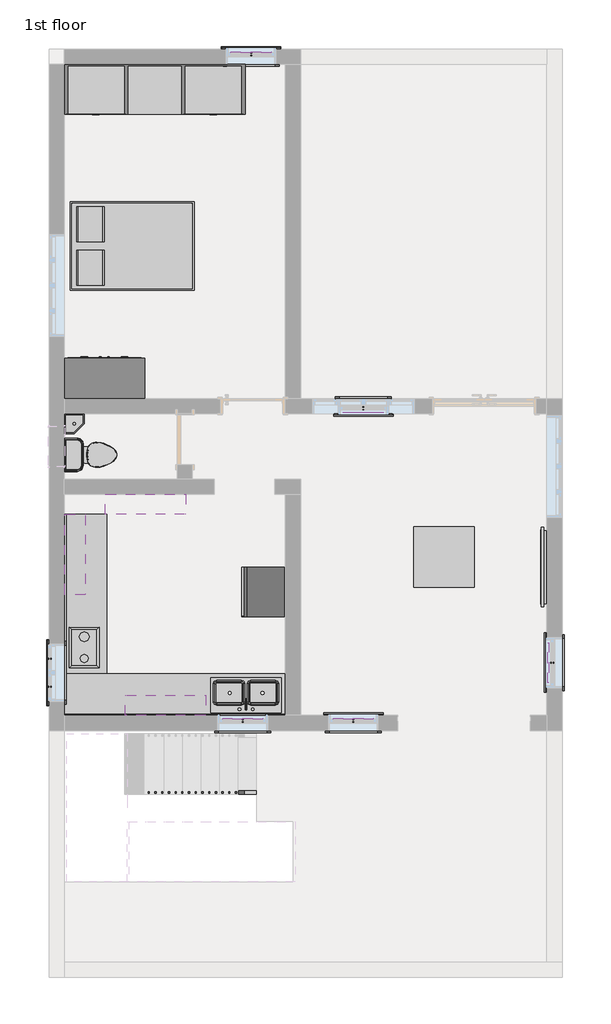
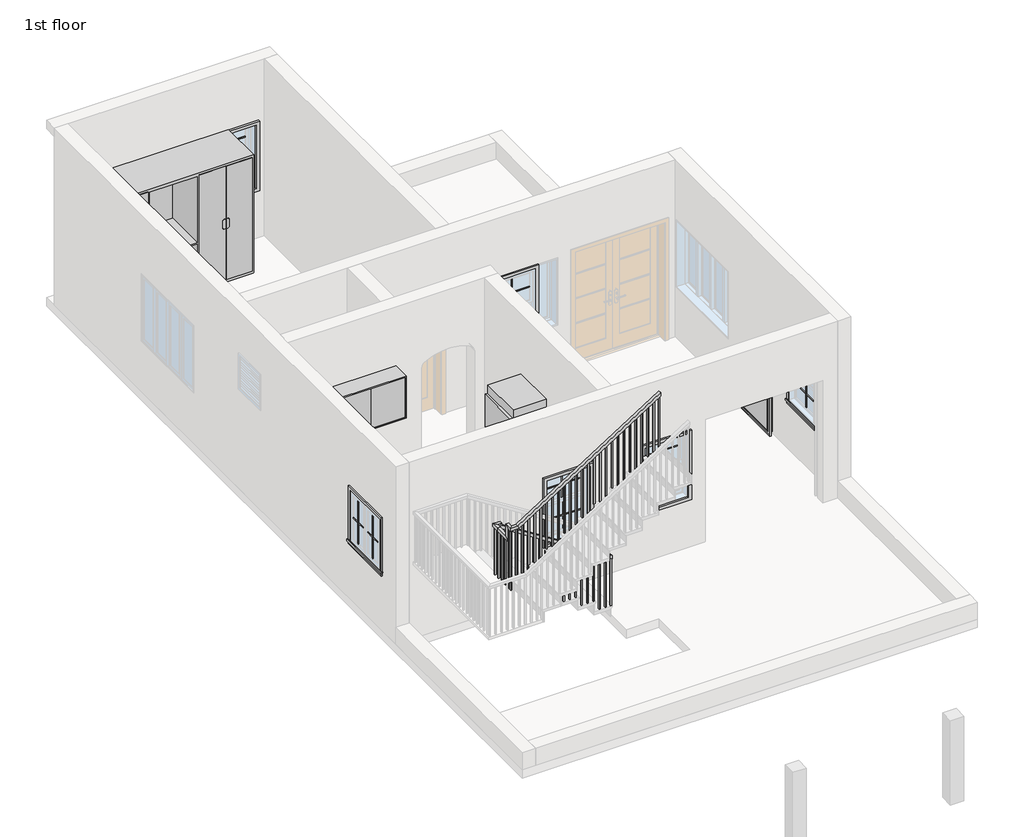
# One storey, part 3 of 3: 26 proxies, 14 furniture elements, 3 flow terminals, 1 railing.
"""IFC4 building model written with IfcOpenShell, lengths in millimetres."""

from ifc_helpers import new_model, si_unit, frame, origin, place, context, project, spatial, polyline, outline, extrude, faceted_brep, transform, mapped, element, save
from components import proxy_3c1fa1d0, muntin_pattern_2x2_muntin_pattern_2x2_b3fe6957, muntin_pattern_2x2_muntin_pattern_2x2_3e0ecaf2, muntin_pattern_2x2_muntin_pattern_2x2_b8ba09c9, muntin_pattern_2x2_muntin_pattern_2x2_d064d722, proxy_76352e5b, trim_window_exterior_flat_with_sill_41619996, trim_window_exterior_flat_with_sill_6cd3ad68, trim_window_exterior_flat_with_sill_e57d6fc0, trim_window_interior_flat_picture_frame_51c85655, trim_window_interior_flat_picture_frame_840a62db, trim_window_interior_flat_picture_frame_50b64344, flow_terminal_080557f2, flow_terminal_a53be723, toilet_domestic_3d_toilet_domestic_3d_ba6479b0, toilet_domestic_3d_toilet_domestic_3d_30431060, furniture_9b4ba0d7, furniture_3428e43d, furniture_97fe820d, furniture_b58f7881, furniture_05b7e736, furniture_e3ff1115, furniture_1f19b6cd, furniture_8a11f05f, furniture_5e39d705, furniture_f491f192, furniture_82e269c4

model = new_model("IFC4")

# Units and contexts
model_context = context("Model", 3, world=origin())
ifc_project = project(units=[si_unit("LENGTHUNIT", "METRE", prefix="MILLI")], contexts=[model_context])

# Site, building, storey
site = spatial("IfcSite", under=ifc_project)
building = spatial("IfcBuilding", under=site)
storey = spatial("IfcBuildingStorey", under=building, Name="1st floor", Elevation=3810.0)

# Proxies
placement = place(None, origin())
proxy_shape = proxy_3c1fa1d0(model_context)
element("IfcBuildingElementProxy", 1, Name="Cook Top-2 Unit : 12\" x 18\" 2", ObjectType="Cook Top-2 Unit : 12\" x 18\" 2", at=placement, inside=storey, context=model_context, shape_type="MappedRepresentation", body=[
    mapped(proxy_shape, transform((28839.5316163, 10560.2732596, 3810.0), x_axis=(1.0, 0.0, 0.0), y_axis=(0.0, 1.0, 0.0), z_axis=(0.0, 0.0, 1.0))),
])
muntin_pattern_2x2_muntin_pattern_2x2_shape = muntin_pattern_2x2_muntin_pattern_2x2_b3fe6957(model_context)
element("IfcBuildingElementProxy", 2, Name="Muntin Pattern_2x2 : Muntin Pattern_2x2", ObjectType="Muntin Pattern_2x2 : Muntin Pattern_2x2", at=placement, inside=storey, context=model_context, shape_type="MappedRepresentation", body=[
    mapped(muntin_pattern_2x2_muntin_pattern_2x2_shape, transform((28391.8566163, 9995.1855552, 4959.35), x_axis=(0.0, 1.0, 0.0), y_axis=(-1.0, 0.0, 0.0), z_axis=(0.0, 0.0, 1.0))),
])
muntin_pattern_2x2_muntin_pattern_2x2_2_shape = muntin_pattern_2x2_muntin_pattern_2x2_3e0ecaf2(model_context)
element("IfcBuildingElementProxy", 3, Name="Muntin Pattern_2x2 : Muntin Pattern_2x2", ObjectType="Muntin Pattern_2x2 : Muntin Pattern_2x2", at=placement, inside=storey, context=model_context, shape_type="MappedRepresentation", body=[
    mapped(muntin_pattern_2x2_muntin_pattern_2x2_2_shape, transform((28391.8566163, 10423.8105552, 4959.35), x_axis=(0.0, -1.0, 0.0), y_axis=(1.0, 0.0, 0.0), z_axis=(0.0, 0.0, 1.0))),
])
muntin_pattern_2x2_muntin_pattern_2x2_3_shape = muntin_pattern_2x2_muntin_pattern_2x2_b8ba09c9(model_context)
element("IfcBuildingElementProxy", 4, Name="Muntin Pattern_2x2 : Muntin Pattern_2x2", ObjectType="Muntin Pattern_2x2 : Muntin Pattern_2x2", at=placement, inside=storey, context=model_context, shape_type="MappedRepresentation", body=[
    mapped(muntin_pattern_2x2_muntin_pattern_2x2_3_shape, transform((32992.4316163, 9526.8730552, 5330.825), x_axis=(1.0, 0.0, 0.0), y_axis=(0.0, 1.0, 0.0), z_axis=(0.0, 0.0, 1.0))),
])
element("IfcBuildingElementProxy", 5, Name="Muntin Pattern_2x2 : Muntin Pattern_2x2", ObjectType="Muntin Pattern_2x2 : Muntin Pattern_2x2", at=placement, inside=storey, context=model_context, shape_type="MappedRepresentation", body=[
    mapped(muntin_pattern_2x2_muntin_pattern_2x2_3_shape, transform((32992.4316163, 9482.4230552, 4800.6), x_axis=(1.0, 0.0, 0.0), y_axis=(0.0, 1.0, 0.0), z_axis=(0.0, 0.0, 1.0))),
])
element("IfcBuildingElementProxy", 6, Name="Muntin Pattern_2x2 : Muntin Pattern_2x2", ObjectType="Muntin Pattern_2x2 : Muntin Pattern_2x2", at=placement, inside=storey, context=model_context, shape_type="MappedRepresentation", body=[
    mapped(muntin_pattern_2x2_muntin_pattern_2x2_3_shape, transform((31316.0316163, 9526.8730552, 5330.825), x_axis=(1.0, 0.0, 0.0), y_axis=(0.0, 1.0, 0.0), z_axis=(0.0, 0.0, 1.0))),
])
element("IfcBuildingElementProxy", 7, Name="Muntin Pattern_2x2 : Muntin Pattern_2x2", ObjectType="Muntin Pattern_2x2 : Muntin Pattern_2x2", at=placement, inside=storey, context=model_context, shape_type="MappedRepresentation", body=[
    mapped(muntin_pattern_2x2_muntin_pattern_2x2_3_shape, transform((31316.0316163, 9482.4230552, 4800.6), x_axis=(1.0, 0.0, 0.0), y_axis=(0.0, 1.0, 0.0), z_axis=(0.0, 0.0, 1.0))),
])
element("IfcBuildingElementProxy", 8, Name="Muntin Pattern_2x2 : Muntin Pattern_2x2", ObjectType="Muntin Pattern_2x2 : Muntin Pattern_2x2", at=placement, inside=storey, context=model_context, shape_type="MappedRepresentation", body=[
    mapped(muntin_pattern_2x2_muntin_pattern_2x2_3_shape, transform((35961.0566163, 10361.8980552, 5330.825), x_axis=(0.0, 1.0, 0.0), y_axis=(-1.0, 0.0, 0.0), z_axis=(0.0, 0.0, 1.0))),
])
element("IfcBuildingElementProxy", 9, Name="Muntin Pattern_2x2 : Muntin Pattern_2x2", ObjectType="Muntin Pattern_2x2 : Muntin Pattern_2x2", at=placement, inside=storey, context=model_context, shape_type="MappedRepresentation", body=[
    mapped(muntin_pattern_2x2_muntin_pattern_2x2_3_shape, transform((36005.5066163, 10361.8980552, 4800.6), x_axis=(0.0, 1.0, 0.0), y_axis=(-1.0, 0.0, 0.0), z_axis=(0.0, 0.0, 1.0))),
])
element("IfcBuildingElementProxy", 10, Name="Muntin Pattern_2x2 : Muntin Pattern_2x2", ObjectType="Muntin Pattern_2x2 : Muntin Pattern_2x2", at=placement, inside=storey, context=model_context, shape_type="MappedRepresentation", body=[
    mapped(muntin_pattern_2x2_muntin_pattern_2x2_3_shape, transform((31443.0316163, 19623.3730552, 5330.825), x_axis=(1.0, 0.0, 0.0), y_axis=(0.0, 1.0, 0.0), z_axis=(0.0, 0.0, 1.0))),
])
element("IfcBuildingElementProxy", 11, Name="Muntin Pattern_2x2 : Muntin Pattern_2x2", ObjectType="Muntin Pattern_2x2 : Muntin Pattern_2x2", at=placement, inside=storey, context=model_context, shape_type="MappedRepresentation", body=[
    mapped(muntin_pattern_2x2_muntin_pattern_2x2_3_shape, transform((31443.0316163, 19578.9230552, 4800.6), x_axis=(1.0, 0.0, 0.0), y_axis=(0.0, 1.0, 0.0), z_axis=(0.0, 0.0, 1.0))),
])
muntin_pattern_2x2_muntin_pattern_2x2_4_shape = muntin_pattern_2x2_muntin_pattern_2x2_d064d722(model_context)
element("IfcBuildingElementProxy", 12, Name="Muntin Pattern_2x2 : Muntin Pattern_2x2", ObjectType="Muntin Pattern_2x2 : Muntin Pattern_2x2", at=placement, inside=storey, context=model_context, shape_type="MappedRepresentation", body=[
    mapped(muntin_pattern_2x2_muntin_pattern_2x2_4_shape, transform((33144.8316163, 14168.7230552, 5330.825), x_axis=(1.0, 0.0, 0.0), y_axis=(0.0, 1.0, 0.0), z_axis=(0.0, 0.0, 1.0))),
])
element("IfcBuildingElementProxy", 13, Name="Muntin Pattern_2x2 : Muntin Pattern_2x2", ObjectType="Muntin Pattern_2x2 : Muntin Pattern_2x2", at=placement, inside=storey, context=model_context, shape_type="MappedRepresentation", body=[
    mapped(muntin_pattern_2x2_muntin_pattern_2x2_4_shape, transform((33144.8316163, 14213.1730552, 4800.6), x_axis=(1.0, 0.0, 0.0), y_axis=(0.0, 1.0, 0.0), z_axis=(0.0, 0.0, 1.0))),
])
proxy_2_shape = proxy_76352e5b(model_context)
element("IfcBuildingElementProxy", 14, Name="Refrigerator-Built-in : 30\" x 24\" LH", ObjectType="Refrigerator-Built-in : 30\" x 24\" LH", at=placement, inside=storey, context=model_context, shape_type="MappedRepresentation", body=[
    mapped(proxy_2_shape, transform((31656.9555878, 11435.0480552, 3810.0), x_axis=(0.0, 1.0, 0.0), y_axis=(-1.0, 0.0, 0.0), z_axis=(0.0, 0.0, 1.0))),
])
trim_window_exterior_flat_with_sill_shape = trim_window_exterior_flat_with_sill_41619996(model_context)
element("IfcBuildingElementProxy", 15, Name="Trim-Window-Exterior-Flat : with Sill", ObjectType="Trim-Window-Exterior-Flat : with Sill", at=placement, inside=storey, context=model_context, shape_type="MappedRepresentation", body=[
    mapped(trim_window_exterior_flat_with_sill_shape, transform((28382.3316163, 10209.4980552, 5803.9), x_axis=(0.0, -1.0, 0.0), y_axis=(0.0, 0.0, 1.0), z_axis=(-1.0, 0.0, 0.0))),
])
trim_window_exterior_flat_with_sill_2_shape = trim_window_exterior_flat_with_sill_6cd3ad68(model_context)
element("IfcBuildingElementProxy", 16, Name="Trim-Window-Exterior-Flat : with Sill", ObjectType="Trim-Window-Exterior-Flat : with Sill", at=placement, inside=storey, context=model_context, shape_type="MappedRepresentation", body=[
    mapped(trim_window_exterior_flat_with_sill_2_shape, transform((32992.4316163, 9561.7980552, 5892.8), x_axis=(-1.0, 0.0, 0.0), y_axis=(0.0, 0.0, 1.0), z_axis=(0.0, 1.0, 0.0))),
])
element("IfcBuildingElementProxy", 17, Name="Trim-Window-Exterior-Flat : with Sill", ObjectType="Trim-Window-Exterior-Flat : with Sill", at=placement, inside=storey, context=model_context, shape_type="MappedRepresentation", body=[
    mapped(trim_window_exterior_flat_with_sill_2_shape, transform((31316.0316163, 9561.7980552, 5892.8), x_axis=(-1.0, 0.0, 0.0), y_axis=(0.0, 0.0, 1.0), z_axis=(0.0, 1.0, 0.0))),
])
element("IfcBuildingElementProxy", 18, Name="Trim-Window-Exterior-Flat : with Sill", ObjectType="Trim-Window-Exterior-Flat : with Sill", at=placement, inside=storey, context=model_context, shape_type="MappedRepresentation", body=[
    mapped(trim_window_exterior_flat_with_sill_2_shape, transform((35926.1316163, 10361.8980552, 5892.8), x_axis=(0.0, -1.0, 0.0), y_axis=(0.0, 0.0, 1.0), z_axis=(-1.0, 0.0, 0.0))),
])
element("IfcBuildingElementProxy", 19, Name="Trim-Window-Exterior-Flat : with Sill", ObjectType="Trim-Window-Exterior-Flat : with Sill", at=placement, inside=storey, context=model_context, shape_type="MappedRepresentation", body=[
    mapped(trim_window_exterior_flat_with_sill_2_shape, transform((31443.0316163, 19658.2980552, 5892.8), x_axis=(-1.0, 0.0, 0.0), y_axis=(0.0, 0.0, 1.0), z_axis=(0.0, 1.0, 0.0))),
])
trim_window_exterior_flat_with_sill_3_shape = trim_window_exterior_flat_with_sill_e57d6fc0(model_context)
element("IfcBuildingElementProxy", 20, Name="Trim-Window-Exterior-Flat : with Sill", ObjectType="Trim-Window-Exterior-Flat : with Sill", at=placement, inside=storey, context=model_context, shape_type="MappedRepresentation", body=[
    mapped(trim_window_exterior_flat_with_sill_3_shape, transform((33144.8316163, 14133.7980552, 5892.8), x_axis=(-1.0, 0.0, 0.0), y_axis=(0.0, 0.0, -1.0), z_axis=(0.0, -1.0, 0.0))),
])
trim_window_interior_flat_picture_frame_shape = trim_window_interior_flat_picture_frame_51c85655(model_context)
element("IfcBuildingElementProxy", 21, Name="Trim-Window-Interior-Flat : Picture Frame", ObjectType="Trim-Window-Interior-Flat : Picture Frame", at=placement, inside=storey, context=model_context, shape_type="MappedRepresentation", body=[
    mapped(trim_window_interior_flat_picture_frame_shape, transform((28610.9316163, 10209.4980552, 5803.9), x_axis=(0.0, 1.0, 0.0), y_axis=(0.0, 0.0, 1.0), z_axis=(1.0, 0.0, 0.0))),
])
trim_window_interior_flat_picture_frame_2_shape = trim_window_interior_flat_picture_frame_840a62db(model_context)
element("IfcBuildingElementProxy", 22, Name="Trim-Window-Interior-Flat : Picture Frame", ObjectType="Trim-Window-Interior-Flat : Picture Frame", at=placement, inside=storey, context=model_context, shape_type="MappedRepresentation", body=[
    mapped(trim_window_interior_flat_picture_frame_2_shape, transform((32992.4316163, 9333.1980552, 5892.8), x_axis=(1.0, 0.0, 0.0), y_axis=(0.0, 0.0, 1.0), z_axis=(0.0, -1.0, 0.0))),
])
element("IfcBuildingElementProxy", 23, Name="Trim-Window-Interior-Flat : Picture Frame", ObjectType="Trim-Window-Interior-Flat : Picture Frame", at=placement, inside=storey, context=model_context, shape_type="MappedRepresentation", body=[
    mapped(trim_window_interior_flat_picture_frame_2_shape, transform((31316.0316163, 9333.1980552, 5892.8), x_axis=(1.0, 0.0, 0.0), y_axis=(0.0, 0.0, 1.0), z_axis=(0.0, -1.0, 0.0))),
])
element("IfcBuildingElementProxy", 24, Name="Trim-Window-Interior-Flat : Picture Frame", ObjectType="Trim-Window-Interior-Flat : Picture Frame", at=placement, inside=storey, context=model_context, shape_type="MappedRepresentation", body=[
    mapped(trim_window_interior_flat_picture_frame_2_shape, transform((36154.7316163, 10361.8980552, 5892.8), x_axis=(0.0, 1.0, 0.0), y_axis=(0.0, 0.0, 1.0), z_axis=(1.0, 0.0, 0.0))),
])
element("IfcBuildingElementProxy", 25, Name="Trim-Window-Interior-Flat : Picture Frame", ObjectType="Trim-Window-Interior-Flat : Picture Frame", at=placement, inside=storey, context=model_context, shape_type="MappedRepresentation", body=[
    mapped(trim_window_interior_flat_picture_frame_2_shape, transform((31443.0316163, 19429.6980552, 5892.8), x_axis=(1.0, 0.0, 0.0), y_axis=(0.0, 0.0, 1.0), z_axis=(0.0, -1.0, 0.0))),
])
trim_window_interior_flat_picture_frame_3_shape = trim_window_interior_flat_picture_frame_50b64344(model_context)
element("IfcBuildingElementProxy", 26, Name="Trim-Window-Interior-Flat : Picture Frame", ObjectType="Trim-Window-Interior-Flat : Picture Frame", at=placement, inside=storey, context=model_context, shape_type="MappedRepresentation", body=[
    mapped(trim_window_interior_flat_picture_frame_3_shape, transform((33144.8316163, 14362.3980552, 5892.8), x_axis=(1.0, 0.0, 0.0), y_axis=(0.0, 0.0, -1.0), z_axis=(0.0, 1.0, 0.0))),
])

# Flow terminals
flow_terminal_shape = flow_terminal_080557f2(model_context)
element("IfcFlowTerminal", 27, ObjectType="Sink - Mop : 28\"x28\" 2", at=placement, inside=storey, context=model_context, shape_type="MappedRepresentation", body=[
    mapped(flow_terminal_shape, transform((28610.9316163, 14133.7980552, 4724.4), x_axis=(1.0, 0.0, 0.0), y_axis=(0.0, 1.0, 0.0), z_axis=(0.0, 0.0, 1.0))),
])
flow_terminal_2_shape = flow_terminal_a53be723(model_context)
element("IfcFlowTerminal", 28, ObjectType="Sink Kitchen-Double : 42\" x 21\"", at=placement, inside=storey, context=model_context, shape_type="MappedRepresentation", body=[
    mapped(flow_terminal_2_shape, transform((31382.5208569, 9868.9434563, 3810.0), x_axis=(-1.0, 0.0, 0.0), y_axis=(0.0, -1.0, 0.0), z_axis=(0.0, 0.0, 1.0))),
])
toilet_domestic_3d_toilet_domestic_3d_shape = toilet_domestic_3d_toilet_domestic_3d_ba6479b0(model_context)
toilet_domestic_3d_toilet_domestic_3d_2_shape = toilet_domestic_3d_toilet_domestic_3d_30431060(model_context)
element("IfcFlowTerminal", 29, ObjectType="Toilet-Domestic-3D : Toilet-Domestic-3D", at=placement, inside=storey, context=model_context, shape_type="MappedRepresentation", body=[
    mapped(toilet_domestic_3d_toilet_domestic_3d_shape, transform((29105.6276437, 13511.4980552, 3810.0), x_axis=(0.0, 1.0, 0.0), y_axis=(-1.0, 0.0, 0.0), z_axis=(0.0, 0.0, 1.0))),
    mapped(toilet_domestic_3d_toilet_domestic_3d_2_shape, transform((29105.6276437, 13511.4980552, 3810.0), x_axis=(0.0, 1.0, 0.0), y_axis=(-1.0, 0.0, 0.0), z_axis=(0.0, 0.0, 1.0))),
])

# Furniture
furniture_shape = furniture_9b4ba0d7(model_context)
element("IfcFurniture", 30, ObjectType="36\"", at=placement, inside=storey, context=model_context, shape_type="MappedRepresentation", body=[
    mapped(furniture_shape, transform((28623.6316163, 12133.8603503, 3810.0), x_axis=(0.0, 1.0, 0.0), y_axis=(-1.0, 0.0, 0.0), z_axis=(0.0, 0.0, 1.0))),
])
furniture_2_shape = furniture_3428e43d(model_context)
element("IfcFurniture", 31, ObjectType="48\"", at=placement, inside=storey, context=model_context, shape_type="MappedRepresentation", body=[
    mapped(furniture_2_shape, transform((30238.4765763, 9561.7980552, 3810.0), x_axis=(-1.0, 0.0, 0.0), y_axis=(0.0, -1.0, 0.0), z_axis=(0.0, 0.0, 1.0))),
])
element("IfcFurniture", 32, ObjectType="48\"", at=placement, inside=storey, context=model_context, shape_type="MappedRepresentation", body=[
    mapped(furniture_2_shape, transform((28623.6316163, 10994.9530952, 3810.0), x_axis=(0.0, 1.0, 0.0), y_axis=(-1.0, 0.0, 0.0), z_axis=(0.0, 0.0, 1.0))),
])
furniture_3_shape = furniture_97fe820d(model_context)
element("IfcFurniture", 33, ObjectType="Base Cabinet-Corner Unit-Square : 36\"", at=placement, inside=storey, context=model_context, shape_type="MappedRepresentation", body=[
    mapped(furniture_3_shape, transform((29150.3693213, 9561.7980552, 3810.0), x_axis=(-1.0, 0.0, 0.0), y_axis=(0.0, -1.0, 0.0), z_axis=(0.0, 0.0, 1.0))),
])
furniture_4_shape = furniture_b58f7881(model_context)
element("IfcFurniture", 34, ObjectType="Bed-Box : Double 53\" x 74\"", at=placement, inside=storey, context=model_context, shape_type="MappedRepresentation", body=[
    mapped(furniture_4_shape, transform((29405.2021081, 16334.6455962, 3810.0), x_axis=(0.0, 1.0, 0.0), y_axis=(-1.0, 0.0, 0.0), z_axis=(0.0, 0.0, 1.0))),
])
furniture_5_shape = furniture_05b7e736(model_context)
element("IfcFurniture", 35, ObjectType="Counter Top : 24\" Depth", at=placement, inside=storey, context=model_context, shape_type="MappedRepresentation", body=[
    mapped(furniture_5_shape, transform((28623.6316163, 11397.2603503, 3810.0), x_axis=(0.0, 1.0, 0.0), y_axis=(-1.0, 0.0, 0.0), z_axis=(0.0, 0.0, 1.0))),
])
furniture_6_shape = furniture_e3ff1115(model_context)
element("IfcFurniture", 36, ObjectType="Counter Top w Sink : 24\" Depth", at=placement, inside=storey, context=model_context, shape_type="MappedRepresentation", body=[
    mapped(furniture_6_shape, transform((30775.9693213, 9561.7980552, 3810.0), x_axis=(-1.0, 0.0, 0.0), y_axis=(0.0, -1.0, 0.0), z_axis=(0.0, 0.0, 1.0))),
])
furniture_7_shape = furniture_1f19b6cd(model_context)
element("IfcFurniture", 37, ObjectType="Entertainment Center.0001 : 96\" x 84\" x 30\"", at=placement, inside=storey, context=model_context, shape_type="MappedRepresentation", body=[
    mapped(furniture_7_shape, transform((29982.5316163, 19455.0980552, 3810.0), x_axis=(1.0, 0.0, 0.0), y_axis=(0.0, 1.0, 0.0), z_axis=(0.0, 0.0, 1.0))),
])
furniture_8_shape = furniture_8a11f05f(model_context)
element("IfcFurniture", 38, ObjectType="Table-Rectangular : 36\" x 36\" 2", at=placement, inside=storey, context=model_context, shape_type="MappedRepresentation", body=[
    mapped(furniture_8_shape, transform((34364.0316163, 11962.0980552, 3810.0), x_axis=(1.0, 0.0, 0.0), y_axis=(0.0, 1.0, 0.0), z_axis=(0.0, 0.0, 1.0))),
])
furniture_9_shape = furniture_5e39d705(model_context)
element("IfcFurniture", 39, ObjectType="Television-Plasma : 50\"", at=placement, inside=storey, context=model_context, shape_type="MappedRepresentation", body=[
    mapped(furniture_9_shape, transform((35926.1316163, 11866.8480552, 3810.0), x_axis=(0.0, -1.0, 0.0), y_axis=(1.0, 0.0, 0.0), z_axis=(0.0, 0.0, 1.0))),
])
furniture_10_shape = furniture_f491f192(model_context)
element("IfcFurniture", 40, ObjectType="Upper Cabinet-Pass-Thru w Glass : 48\" x 30\" x 12\"", at=placement, inside=storey, context=model_context, shape_type="MappedRepresentation", body=[
    mapped(furniture_10_shape, transform((28623.6316163, 11981.4603503, 3810.0), x_axis=(0.0, 1.0, 0.0), y_axis=(-1.0, 0.0, 0.0), z_axis=(0.0, 0.0, 1.0))),
])
element("IfcFurniture", 41, ObjectType="Upper Cabinet-Pass-Thru w Glass : 48\" x 30\" x 12\"", at=placement, inside=storey, context=model_context, shape_type="MappedRepresentation", body=[
    mapped(furniture_10_shape, transform((29861.5693213, 12609.7980552, 3810.0), x_axis=(-1.0, 0.0, 0.0), y_axis=(0.0, -1.0, 0.0), z_axis=(0.0, 0.0, 1.0))),
])
element("IfcFurniture", 42, ObjectType="Upper Cabinet-Pass-Thru w Glass : 48\" x 30\" x 12\"", at=placement, inside=storey, context=model_context, shape_type="MappedRepresentation", body=[
    mapped(furniture_10_shape, transform((30166.3693213, 9561.7980552, 3810.0), x_axis=(-1.0, 0.0, 0.0), y_axis=(0.0, -1.0, 0.0), z_axis=(0.0, 0.0, 1.0))),
])
furniture_11_shape = furniture_82e269c4(model_context)
element("IfcFurniture", 43, ObjectType="Wardrobe : 48\" x 72\" x 24\"", at=placement, inside=storey, context=model_context, shape_type="MappedRepresentation", body=[
    mapped(furniture_11_shape, transform((28951.3383565, 14083.4592456, 3810.0), x_axis=(-1.0, 0.0, 0.0), y_axis=(0.0, -1.0, 0.0), z_axis=(0.0, 0.0, 1.0))),
])

# Railing
element("IfcRailing", 44, ObjectType="Handrail - Rectangular", at=placement, inside=storey, context=model_context, shape_type="SolidModel", body=[
    faceted_brep([(31519.2316163, 8367.9980552, 4902.2), (31519.2316163, 8367.9980552, 4841.986276), (31519.2316163, 8418.7980552, 4841.986276), (31519.2316163, 8418.7980552, 4902.2), (29639.6316163, 8367.9980552, 6098.3090909), (29588.8316163, 8367.9980552, 6070.4226396), (29588.8316163, 8418.7980552, 6070.4226396), (29639.6316163, 8418.7980552, 6098.3090909), (29639.6316163, 8367.9980552, 6146.8), (29588.8316163, 8367.9980552, 6096.0), (29588.8316163, 8418.7980552, 6096.0), (29639.6316163, 8418.7980552, 6146.8), (29563.4316163, 8367.9980552, 6146.8), (29563.4316163, 8367.9980552, 6096.0), (29512.6316163, 8418.7980552, 6096.0), (29512.6316163, 8418.7980552, 6146.8), (29563.4316163, 8291.7980552, 6146.8), (29563.4316163, 8291.7980552, 6096.0), (29512.6316163, 8291.7980552, 6096.0), (29512.6316163, 8291.7980552, 6146.8), (29563.4316163, 8031.4480552, 6146.8), (29563.4316163, 7980.6480552, 6096.0), (29512.6316163, 7980.6480552, 6096.0), (29512.6316163, 8031.4480552, 6146.8), (29563.4316163, 8031.4480552, 6373.0909091), (29563.4316163, 7980.6480552, 6322.2909091), (29512.6316163, 7980.6480552, 6322.2909091), (29512.6316163, 8031.4480552, 6373.0909091), (29563.4316163, 7955.2480552, 6373.0909091), (29563.4316163, 7955.2480552, 6322.2909091), (29512.6316163, 7904.4480552, 6322.2909091), (29512.6316163, 7904.4480552, 6373.0909091), (29639.6316163, 7955.2480552, 6373.0909091), (29654.4246113, 7955.2480552, 6322.2909091), (29654.4246113, 7904.4480552, 6322.2909091), (29639.6316163, 7904.4480552, 6373.0909091), (32078.0316163, 7955.2480552, 7924.8), (32078.0316163, 7904.4480552, 7924.8), (32078.0316163, 7904.4480552, 7864.586276), (32078.0316163, 7955.2480552, 7864.586276)], [[[0, 1, 2, 3]], [[1, 0, 4, 5]], [[2, 1, 5, 6]], [[3, 2, 6, 7]], [[0, 3, 7, 4]], [[5, 4, 8, 9]], [[6, 5, 9, 10]], [[7, 6, 10, 11]], [[4, 7, 11, 8]], [[9, 8, 12, 13]], [[10, 9, 13, 14]], [[11, 10, 14, 15]], [[8, 11, 15, 12]], [[13, 12, 16, 17]], [[14, 13, 17, 18]], [[15, 14, 18, 19]], [[12, 15, 19, 16]], [[17, 16, 20, 21]], [[18, 17, 21, 22]], [[19, 18, 22, 23]], [[16, 19, 23, 20]], [[21, 20, 24, 25]], [[22, 21, 25, 26]], [[23, 22, 26, 27]], [[20, 23, 27, 24]], [[25, 24, 28, 29]], [[26, 25, 29, 30]], [[27, 26, 30, 31]], [[24, 27, 31, 28]], [[29, 28, 32, 33]], [[30, 29, 33, 34]], [[31, 30, 34, 35]], [[28, 31, 35, 32]], [[36, 37, 38, 39]], [[33, 32, 36, 39]], [[34, 33, 39, 38]], [[35, 34, 38, 37]], [[32, 35, 37, 36]]]),
    extrude(outline(polyline([(7793.8703669, 31966.9066163), (6832.6, 31966.9066163), (6832.6, 31985.9566163), (7805.9930941, 31985.9566163), (7793.8703669, 31966.9066163)])), frame((0.0, 7920.3230552, 0.0), z_axis=(0.0, 1.0, 0.0), x_axis=(0.0, 0.0, 1.0)), (0.0, 0.0, 1.0), 19.05),
    extrude(outline(polyline([(7729.2158214, 31865.3066163), (6832.6, 31865.3066163), (6832.6, 31884.3566163), (7741.3385487, 31884.3566163), (7729.2158214, 31865.3066163)])), frame((0.0, 7920.3230552, 0.0), z_axis=(0.0, 1.0, 0.0), x_axis=(0.0, 0.0, 1.0)), (0.0, 0.0, 1.0), 19.05),
    extrude(outline(polyline([(7664.561276, 31763.7066163), (6654.8, 31763.7066163), (6654.8, 31782.7566163), (7676.6840032, 31782.7566163), (7664.561276, 31763.7066163)])), frame((0.0, 7920.3230552, 0.0), z_axis=(0.0, 1.0, 0.0), x_axis=(0.0, 0.0, 1.0)), (0.0, 0.0, 1.0), 19.05),
    extrude(outline(polyline([(7599.9067305, 31662.1066163), (6654.8, 31662.1066163), (6654.8, 31681.1566163), (7612.0294578, 31681.1566163), (7599.9067305, 31662.1066163)])), frame((0.0, 7920.3230552, 0.0), z_axis=(0.0, 1.0, 0.0), x_axis=(0.0, 0.0, 1.0)), (0.0, 0.0, 1.0), 19.05),
    extrude(outline(polyline([(7535.2521851, 31560.5066163), (6654.8, 31560.5066163), (6654.8, 31579.5566163), (7547.3749123, 31579.5566163), (7535.2521851, 31560.5066163)])), frame((0.0, 7920.3230552, 0.0), z_axis=(0.0, 1.0, 0.0), x_axis=(0.0, 0.0, 1.0)), (0.0, 0.0, 1.0), 19.05),
    extrude(outline(polyline([(7470.5976396, 31458.9066163), (6477.0, 31458.9066163), (6477.0, 31477.9566163), (7482.7203669, 31477.9566163), (7470.5976396, 31458.9066163)])), frame((0.0, 7920.3230552, 0.0), z_axis=(0.0, 1.0, 0.0), x_axis=(0.0, 0.0, 1.0)), (0.0, 0.0, 1.0), 19.05),
    extrude(outline(polyline([(7405.9430941, 31357.3066163), (6477.0, 31357.3066163), (6477.0, 31376.3566163), (7418.0658214, 31376.3566163), (7405.9430941, 31357.3066163)])), frame((0.0, 7920.3230552, 0.0), z_axis=(0.0, 1.0, 0.0), x_axis=(0.0, 0.0, 1.0)), (0.0, 0.0, 1.0), 19.05),
    extrude(outline(polyline([(7341.2885487, 31255.7066163), (6477.0, 31255.7066163), (6477.0, 31274.7566163), (7353.411276, 31274.7566163), (7341.2885487, 31255.7066163)])), frame((0.0, 7920.3230552, 0.0), z_axis=(0.0, 1.0, 0.0), x_axis=(0.0, 0.0, 1.0)), (0.0, 0.0, 1.0), 19.05),
    extrude(outline(polyline([(7276.6340032, 31154.1066163), (6299.2, 31154.1066163), (6299.2, 31173.1566163), (7288.7567305, 31173.1566163), (7276.6340032, 31154.1066163)])), frame((0.0, 7920.3230552, 0.0), z_axis=(0.0, 1.0, 0.0), x_axis=(0.0, 0.0, 1.0)), (0.0, 0.0, 1.0), 19.05),
    extrude(outline(polyline([(7211.9794578, 31052.5066163), (6299.2, 31052.5066163), (6299.2, 31071.5566163), (7224.1021851, 31071.5566163), (7211.9794578, 31052.5066163)])), frame((0.0, 7920.3230552, 0.0), z_axis=(0.0, 1.0, 0.0), x_axis=(0.0, 0.0, 1.0)), (0.0, 0.0, 1.0), 19.05),
    extrude(outline(polyline([(7147.3249123, 30950.9066163), (6299.2, 30950.9066163), (6299.2, 30969.9566163), (7159.4476396, 30969.9566163), (7147.3249123, 30950.9066163)])), frame((0.0, 7920.3230552, 0.0), z_axis=(0.0, 1.0, 0.0), x_axis=(0.0, 0.0, 1.0)), (0.0, 0.0, 1.0), 19.05),
    extrude(outline(polyline([(7082.6703669, 30849.3066163), (6121.4, 30849.3066163), (6121.4, 30868.3566163), (7094.7930941, 30868.3566163), (7082.6703669, 30849.3066163)])), frame((0.0, 7920.3230552, 0.0), z_axis=(0.0, 1.0, 0.0), x_axis=(0.0, 0.0, 1.0)), (0.0, 0.0, 1.0), 19.05),
    extrude(outline(polyline([(7018.0158214, 30747.7066163), (6121.4, 30747.7066163), (6121.4, 30766.7566163), (7030.1385487, 30766.7566163), (7018.0158214, 30747.7066163)])), frame((0.0, 7920.3230552, 0.0), z_axis=(0.0, 1.0, 0.0), x_axis=(0.0, 0.0, 1.0)), (0.0, 0.0, 1.0), 19.05),
    extrude(outline(polyline([(6953.361276, 30646.1066163), (5943.6, 30646.1066163), (5943.6, 30665.1566163), (6965.4840032, 30665.1566163), (6953.361276, 30646.1066163)])), frame((0.0, 7920.3230552, 0.0), z_axis=(0.0, 1.0, 0.0), x_axis=(0.0, 0.0, 1.0)), (0.0, 0.0, 1.0), 19.05),
    extrude(outline(polyline([(6888.7067305, 30544.5066163), (5943.6, 30544.5066163), (5943.6, 30563.5566163), (6900.8294578, 30563.5566163), (6888.7067305, 30544.5066163)])), frame((0.0, 7920.3230552, 0.0), z_axis=(0.0, 1.0, 0.0), x_axis=(0.0, 0.0, 1.0)), (0.0, 0.0, 1.0), 19.05),
    extrude(outline(polyline([(6824.0521851, 30442.9066163), (5943.6, 30442.9066163), (5943.6, 30461.9566163), (6836.1749123, 30461.9566163), (6824.0521851, 30442.9066163)])), frame((0.0, 7920.3230552, 0.0), z_axis=(0.0, 1.0, 0.0), x_axis=(0.0, 0.0, 1.0)), (0.0, 0.0, 1.0), 19.05),
    extrude(outline(polyline([(6759.3976396, 30341.3066163), (5765.8, 30341.3066163), (5765.8, 30360.3566163), (6771.5203669, 30360.3566163), (6759.3976396, 30341.3066163)])), frame((0.0, 7920.3230552, 0.0), z_axis=(0.0, 1.0, 0.0), x_axis=(0.0, 0.0, 1.0)), (0.0, 0.0, 1.0), 19.05),
    extrude(outline(polyline([(6694.7430941, 30239.7066163), (5765.8, 30239.7066163), (5765.8, 30258.7566163), (6706.8658214, 30258.7566163), (6694.7430941, 30239.7066163)])), frame((0.0, 7920.3230552, 0.0), z_axis=(0.0, 1.0, 0.0), x_axis=(0.0, 0.0, 1.0)), (0.0, 0.0, 1.0), 19.05),
    extrude(outline(polyline([(6630.0885487, 30138.1066163), (5765.8, 30138.1066163), (5765.8, 30157.1566163), (6642.211276, 30157.1566163), (6630.0885487, 30138.1066163)])), frame((0.0, 7920.3230552, 0.0), z_axis=(0.0, 1.0, 0.0), x_axis=(0.0, 0.0, 1.0)), (0.0, 0.0, 1.0), 19.05),
    extrude(outline(polyline([(6565.4340032, 30036.5066163), (5588.0, 30036.5066163), (5588.0, 30055.5566163), (6577.5567305, 30055.5566163), (6565.4340032, 30036.5066163)])), frame((0.0, 7920.3230552, 0.0), z_axis=(0.0, 1.0, 0.0), x_axis=(0.0, 0.0, 1.0)), (0.0, 0.0, 1.0), 19.05),
    extrude(outline(polyline([(6500.7794578, 29934.9066163), (5588.0, 29934.9066163), (5588.0, 29953.9566163), (6512.9021851, 29953.9566163), (6500.7794578, 29934.9066163)])), frame((0.0, 7920.3230552, 0.0), z_axis=(0.0, 1.0, 0.0), x_axis=(0.0, 0.0, 1.0)), (0.0, 0.0, 1.0), 19.05),
    extrude(outline(polyline([(6436.1249123, 29833.3066163), (5588.0, 29833.3066163), (5588.0, 29852.3566163), (6448.2476396, 29852.3566163), (6436.1249123, 29833.3066163)])), frame((0.0, 7920.3230552, 0.0), z_axis=(0.0, 1.0, 0.0), x_axis=(0.0, 0.0, 1.0)), (0.0, 0.0, 1.0), 19.05),
    extrude(outline(polyline([(6371.4703669, 29731.7066163), (5410.2, 29731.7066163), (5410.2, 29750.7566163), (6383.5930941, 29750.7566163), (6371.4703669, 29731.7066163)])), frame((0.0, 7920.3230552, 0.0), z_axis=(0.0, 1.0, 0.0), x_axis=(0.0, 0.0, 1.0)), (0.0, 0.0, 1.0), 19.05),
    extrude(outline(polyline([(6306.8158214, 29630.1066163), (5410.2, 29630.1066163), (5410.2, 29649.1566163), (6318.9385487, 29649.1566163), (6306.8158214, 29630.1066163)])), frame((0.0, 7920.3230552, 0.0), z_axis=(0.0, 1.0, 0.0), x_axis=(0.0, 0.0, 1.0)), (0.0, 0.0, 1.0), 19.05),
    extrude(outline(polyline([(29547.5566163, 7996.5230552), (29547.5566163, 7977.4730552), (29528.5066163, 7977.4730552), (29528.5066163, 7996.5230552), (29547.5566163, 7996.5230552)])), frame((0.0, 0.0, 5232.4), z_axis=(0.0, 0.0, 1.0), x_axis=(1.0, 0.0, 0.0)), (0.0, 0.0, 1.0), 1089.8909091),
    extrude(outline(polyline([(29547.5566163, 8098.1230552), (29547.5566163, 8079.0730552), (29528.5066163, 8079.0730552), (29528.5066163, 8098.1230552), (29547.5566163, 8098.1230552)])), frame((0.0, 0.0, 5232.4), z_axis=(0.0, 0.0, 1.0), x_axis=(1.0, 0.0, 0.0)), (0.0, 0.0, 1.0), 863.6),
    extrude(outline(polyline([(29547.5566163, 8199.7230552), (29547.5566163, 8180.6730552), (29528.5066163, 8180.6730552), (29528.5066163, 8199.7230552), (29547.5566163, 8199.7230552)])), frame((0.0, 0.0, 5232.4), z_axis=(0.0, 0.0, 1.0), x_axis=(1.0, 0.0, 0.0)), (0.0, 0.0, 1.0), 863.6),
    extrude(outline(polyline([(29547.5566163, 8301.3230552), (29547.5566163, 8282.2730552), (29528.5066163, 8282.2730552), (29528.5066163, 8301.3230552), (29547.5566163, 8301.3230552)])), frame((0.0, 0.0, 5232.4), z_axis=(0.0, 0.0, 1.0), x_axis=(1.0, 0.0, 0.0)), (0.0, 0.0, 1.0), 863.6),
    extrude(outline(polyline([(29598.3566163, 8383.8730552), (29579.3066163, 8383.8730552), (29579.3066163, 8402.9230552), (29598.3566163, 8402.9230552), (29598.3566163, 8383.8730552)])), frame((0.0, 0.0, 5054.6), z_axis=(0.0, 0.0, 1.0), x_axis=(1.0, 0.0, 0.0)), (0.0, 0.0, 1.0), 1041.4),
    extrude(outline(polyline([(6011.8294578, 29680.9066163), (5054.6, 29680.9066163), (5054.6, 29699.9566163), (5999.7067305, 29699.9566163), (6011.8294578, 29680.9066163)])), frame((0.0, 8383.8730552, 0.0), z_axis=(0.0, 1.0, 0.0), x_axis=(0.0, 0.0, 1.0)), (0.0, 0.0, 1.0), 19.05),
    extrude(outline(polyline([(5947.1749123, 29782.5066163), (5054.6, 29782.5066163), (5054.6, 29801.5566163), (5935.0521851, 29801.5566163), (5947.1749123, 29782.5066163)])), frame((0.0, 8383.8730552, 0.0), z_axis=(0.0, 1.0, 0.0), x_axis=(0.0, 0.0, 1.0)), (0.0, 0.0, 1.0), 19.05),
    extrude(outline(polyline([(5882.5203669, 29884.1066163), (4876.8, 29884.1066163), (4876.8, 29903.1566163), (5870.3976396, 29903.1566163), (5882.5203669, 29884.1066163)])), frame((0.0, 8383.8730552, 0.0), z_axis=(0.0, 1.0, 0.0), x_axis=(0.0, 0.0, 1.0)), (0.0, 0.0, 1.0), 19.05),
    extrude(outline(polyline([(5817.8658214, 29985.7066163), (4876.8, 29985.7066163), (4876.8, 30004.7566163), (5805.7430941, 30004.7566163), (5817.8658214, 29985.7066163)])), frame((0.0, 8383.8730552, 0.0), z_axis=(0.0, 1.0, 0.0), x_axis=(0.0, 0.0, 1.0)), (0.0, 0.0, 1.0), 19.05),
    extrude(outline(polyline([(5753.211276, 30087.3066163), (4876.8, 30087.3066163), (4876.8, 30106.3566163), (5741.0885487, 30106.3566163), (5753.211276, 30087.3066163)])), frame((0.0, 8383.8730552, 0.0), z_axis=(0.0, 1.0, 0.0), x_axis=(0.0, 0.0, 1.0)), (0.0, 0.0, 1.0), 19.05),
    extrude(outline(polyline([(5688.5567305, 30188.9066163), (4699.0, 30188.9066163), (4699.0, 30207.9566163), (5676.4340032, 30207.9566163), (5688.5567305, 30188.9066163)])), frame((0.0, 8383.8730552, 0.0), z_axis=(0.0, 1.0, 0.0), x_axis=(0.0, 0.0, 1.0)), (0.0, 0.0, 1.0), 19.05),
    extrude(outline(polyline([(5623.9021851, 30290.5066163), (4699.0, 30290.5066163), (4699.0, 30309.5566163), (5611.7794578, 30309.5566163), (5623.9021851, 30290.5066163)])), frame((0.0, 8383.8730552, 0.0), z_axis=(0.0, 1.0, 0.0), x_axis=(0.0, 0.0, 1.0)), (0.0, 0.0, 1.0), 19.05),
    extrude(outline(polyline([(5559.2476396, 30392.1066163), (4699.0, 30392.1066163), (4699.0, 30411.1566163), (5547.1249123, 30411.1566163), (5559.2476396, 30392.1066163)])), frame((0.0, 8383.8730552, 0.0), z_axis=(0.0, 1.0, 0.0), x_axis=(0.0, 0.0, 1.0)), (0.0, 0.0, 1.0), 19.05),
    extrude(outline(polyline([(5494.5930941, 30493.7066163), (4521.2, 30493.7066163), (4521.2, 30512.7566163), (5482.4703669, 30512.7566163), (5494.5930941, 30493.7066163)])), frame((0.0, 8383.8730552, 0.0), z_axis=(0.0, 1.0, 0.0), x_axis=(0.0, 0.0, 1.0)), (0.0, 0.0, 1.0), 19.05),
    extrude(outline(polyline([(5429.9385487, 30595.3066163), (4521.2, 30595.3066163), (4521.2, 30614.3566163), (5417.8158214, 30614.3566163), (5429.9385487, 30595.3066163)])), frame((0.0, 8383.8730552, 0.0), z_axis=(0.0, 1.0, 0.0), x_axis=(0.0, 0.0, 1.0)), (0.0, 0.0, 1.0), 19.05),
    extrude(outline(polyline([(5365.2840032, 30696.9066163), (4343.4, 30696.9066163), (4343.4, 30715.9566163), (5353.161276, 30715.9566163), (5365.2840032, 30696.9066163)])), frame((0.0, 8383.8730552, 0.0), z_axis=(0.0, 1.0, 0.0), x_axis=(0.0, 0.0, 1.0)), (0.0, 0.0, 1.0), 19.05),
    extrude(outline(polyline([(5300.6294578, 30798.5066163), (4343.4, 30798.5066163), (4343.4, 30817.5566163), (5288.5067305, 30817.5566163), (5300.6294578, 30798.5066163)])), frame((0.0, 8383.8730552, 0.0), z_axis=(0.0, 1.0, 0.0), x_axis=(0.0, 0.0, 1.0)), (0.0, 0.0, 1.0), 19.05),
    extrude(outline(polyline([(5235.9749123, 30900.1066163), (4343.4, 30900.1066163), (4343.4, 30919.1566163), (5223.8521851, 30919.1566163), (5235.9749123, 30900.1066163)])), frame((0.0, 8383.8730552, 0.0), z_axis=(0.0, 1.0, 0.0), x_axis=(0.0, 0.0, 1.0)), (0.0, 0.0, 1.0), 19.05),
    extrude(outline(polyline([(5171.3203669, 31001.7066163), (4165.6, 31001.7066163), (4165.6, 31020.7566163), (5159.1976396, 31020.7566163), (5171.3203669, 31001.7066163)])), frame((0.0, 8383.8730552, 0.0), z_axis=(0.0, 1.0, 0.0), x_axis=(0.0, 0.0, 1.0)), (0.0, 0.0, 1.0), 19.05),
    extrude(outline(polyline([(5106.6658214, 31103.3066163), (4165.6, 31103.3066163), (4165.6, 31122.3566163), (5094.5430941, 31122.3566163), (5106.6658214, 31103.3066163)])), frame((0.0, 8383.8730552, 0.0), z_axis=(0.0, 1.0, 0.0), x_axis=(0.0, 0.0, 1.0)), (0.0, 0.0, 1.0), 19.05),
    extrude(outline(polyline([(5042.011276, 31204.9066163), (4165.6, 31204.9066163), (4165.6, 31223.9566163), (5029.8885487, 31223.9566163), (5042.011276, 31204.9066163)])), frame((0.0, 8383.8730552, 0.0), z_axis=(0.0, 1.0, 0.0), x_axis=(0.0, 0.0, 1.0)), (0.0, 0.0, 1.0), 19.05),
    extrude(outline(polyline([(4977.3567305, 31306.5066163), (3987.8, 31306.5066163), (3987.8, 31325.5566163), (4965.2340032, 31325.5566163), (4977.3567305, 31306.5066163)])), frame((0.0, 8383.8730552, 0.0), z_axis=(0.0, 1.0, 0.0), x_axis=(0.0, 0.0, 1.0)), (0.0, 0.0, 1.0), 19.05),
    extrude(outline(polyline([(4912.7021851, 31408.1066163), (3987.8, 31408.1066163), (3987.8, 31427.1566163), (4900.5794578, 31427.1566163), (4912.7021851, 31408.1066163)])), frame((0.0, 8383.8730552, 0.0), z_axis=(0.0, 1.0, 0.0), x_axis=(0.0, 0.0, 1.0)), (0.0, 0.0, 1.0), 19.05),
    extrude(outline(polyline([(29547.5566163, 7939.3730552), (29547.5566163, 7920.3230552), (29528.5066163, 7920.3230552), (29528.5066163, 7939.3730552), (29547.5566163, 7939.3730552)])), frame((0.0, 0.0, 5232.4), z_axis=(0.0, 0.0, 1.0), x_axis=(1.0, 0.0, 0.0)), (0.0, 0.0, 1.0), 1089.8909091),
    extrude(outline(polyline([(29547.5566163, 8383.8730552), (29528.5066163, 8383.8730552), (29528.5066163, 8402.9230552), (29547.5566163, 8402.9230552), (29547.5566163, 8383.8730552)])), frame((0.0, 0.0, 5232.4), z_axis=(0.0, 0.0, 1.0), x_axis=(1.0, 0.0, 0.0)), (0.0, 0.0, 1.0), 863.6),
    extrude(outline(polyline([(7852.4635487, 32058.9816163), (6832.6, 32058.9816163), (6832.6, 32078.0316163), (7864.586276, 32078.0316163), (7852.4635487, 32058.9816163)])), frame((0.0, 7920.3230552, 0.0), z_axis=(0.0, 1.0, 0.0), x_axis=(0.0, 0.0, 1.0)), (0.0, 0.0, 1.0), 19.05),
    extrude(outline(polyline([(4854.1090032, 31500.1816163), (3987.8, 31500.1816163), (3987.8, 31519.2316163), (4841.986276, 31519.2316163), (4854.1090032, 31500.1816163)])), frame((0.0, 8383.8730552, 0.0), z_axis=(0.0, 1.0, 0.0), x_axis=(0.0, 0.0, 1.0)), (0.0, 0.0, 1.0), 19.05),
])

save(model, "model.ifc")

# Revit data of these elements
# Type "Cook Top-2 Unit : 12\" x 18\" 2"
#   Assembly Code = "E1090400"
#   Counter Height = 3' - 0"
#   Depth = 2' - 0"
#   Width = 1' - 6"
#   Burner Material = Metal - Chrome
#   Cooktop Material = Metal - Steel, Polished
#   Default Elevation = 0
# Type "Muntin Pattern_2x2 : Muntin Pattern_2x2"
#   Width [instance default] = 4' - 0"
#   Thickness = 0' - 0 1/2"
#   Height [instance default] = 4' - 0"
#   Distance = 0' - 0 3/4"
#   Interior Material [instance default] = none
#   Exterior Material [instance default] = none
#   Default Elevation = 0
# Type "Refrigerator-Built-in : 30\" x 24\" LH"
#   Assembly Code = "E1090400"
#   Depth = 2' - 0"
#   Handle = 0' - 0 1/4"
#   Height = 7' - 0"
#   Top Door Height = 5' - 0"
#   Width = 2' - 5 1/2"
#   Material = Metal - Paint Finish - Ivory,Glossy
#   Default Elevation = 0
# Type "Trim-Window-Exterior-Flat : with Sill"
#   Trim Width = 0' - 2 1/4"
#   Trim Thickness_Picture Frame = 0' - 1 1/4"
#   Trim Thickness_with Sill = 0' - 0 3/4"
#   Sill Thickness = 0' - 1 1/4"
#   Opening Width [instance default] = 2' - 0"
#   Opening Height [instance default] = 3' - 0"
#   Default Elevation = 4' - 0"
#   Sill = yes
#   Picture Frame = no
#   Trim Material [instance default] = none
# Type "Trim-Window-Interior-Flat : Picture Frame"
#   Trim Thickness_Picture Frame = 0' - 1 1/4"
#   Trim Width = 0' - 2 1/4"
#   Trim Thickness_with Sill = 0' - 0 3/4"
#   Sill Thickness = 0' - 1 1/4"
#   Opening Width [instance default] = 2' - 0"
#   Opening Height [instance default] = 3' - 0"
#   Default Elevation = 4' - 0"
#   Sill = no
#   Picture Frame = yes
#   Trim Material [instance default] = none
# Type "Sink - Mop : 28\"x28\" 2"
#   WFU = 2
#   Sink Width = 1' - 0"
#   Sink Length = 1' - 0"
#   Sanitary Radius = 1"
#   Sanitary Diameter = 2"
#   Half Sink Width = 0' - 6"
#   Half Sink Length = 0' - 6"
#   Sink Material = none
#   HWFU = 0
#   Default Elevation = 0
#   CWFU = 0
#   Assembly Code = ""
# Type "Sink Kitchen-Double : 42\" x 21\""
#   Assembly Code = "D2010410"
#   Counter Height = 3' - 0"
#   Depth = 1' - 9"
#   Width = 3' - 6"
#   Faucet Material = Steel, Polished
#   Sink Material = Steel, Polished
#   Default Elevation = 0
# Type "Toilet-Domestic-3D : Toilet-Domestic-3D"
#   Assembly Code = "D2010110"
#   Toilet - Bowl/Basin Material = Porcelain, Linen
#   Toilet - Seat Material = Laminate, Linen, Matte
#   Default Elevation = 0
# Type "36\""
#   Assembly Code = "C1030410"
#   Depth = 2' - 0"
#   Height = 2' - 10 1/2"
#   Toe Depth = 0' - 3"
#   Toe Height = 0' - 3 1/2"
#   Width = 3' - 0"
#   Cabinet Material = Cabinets
#   Door/Drawer Material = Cabinets
#   Handle Material = Cabinets - Handles
#   Default Elevation = 0
# Type "48\""
#   Assembly Code = "C1030410"
#   Depth = 2' - 0"
#   Height = 2' - 10 1/2"
#   Toe Depth = 0' - 3"
#   Toe Height = 0' - 3 1/2"
#   Width = 4' - 0"
#   Cabinet Material = none
#   Door/Drawer Material = none
#   Handle Material = Cabinets - Handles
#   Default Elevation = 0
# Type "Base Cabinet-Corner Unit-Square : 36\""
#   Assembly Code = "C1030410"
#   Depth = 2' - 0"
#   Height = 2' - 10 1/2"
#   Toe Depth = 0' - 3"
#   Toe Height = 0' - 3 1/2"
#   Width = 3' - 0"
#   Cabinet Material = Cabinets
#   Door/Drawer Material = Cabinets
#   Handle Material = Cabinets - Handles
#   Default Elevation = 0
# Type "Bed-Box : Double 53\" x 74\""
#   Assembly Code = "E2020200"
#   Length = 6' - 2"
#   Width = 4' - 5"
#   Frame Material = Birch
#   Mattress Material = Linen, White
#   Default Elevation = 0
# Type "Counter Top : 24\" Depth"
#   Assembly Code = "C1030400"
#   Counter Thickness = 0' - 1 1/2"
#   Depth = 2' - 1"
#   Height = 3' - 0"
#   Length [instance default] = 8' - 0"
#   Counter Top Material = none
#   Default Elevation = 0
# Type "Counter Top w Sink : 24\" Depth"
#   Assembly Code = "C1030400"
#   Counter Thickness = 0' - 1 1/2"
#   Depth = 2' - 1"
#   Height = 3' - 0"
#   Length [instance default] = 8' - 0"
#   Sink Location [instance default] = 2' - 0"
#   Sink Location To Wall [instance default] = 0' - 6"
#   Sink Opening Depth [instance default] = 1' - 3"
#   Sink Opening Width [instance default] = 3' - 3"
#   Counter Top Material = none
#   Default Elevation = 0
# Type "Entertainment Center.0001 : 96\" x 84\" x 30\""
#   Assembly Code = "E2020200"
#   Center Width = 2' - 8"
#   Depth = 2' - 6"
#   Height = 7' - 0"
#   Width = 9' - 0"
#   Material = Laminate, Ivory, Matte
#   Default Elevation = 0
# Type "Table-Rectangular : 36\" x 36\" 2"
#   Assembly Code = "E2020200"
#   Height = 1' - 6"
#   Length = 3' - 0"
#   Width = 3' - 0"
#   Base Material = Birch
#   Top Material = Birch
#   Default Elevation = 0
# Type "Television-Plasma : 50\""
#   Assembly Code = "E2020200"
#   Depth = 0' - 3 1/2"
#   Height = 2' - 6"
#   Width = 3' - 11 1/2"
#   Cabinet Material = Plastic - Gray
#   Default Elevation = 0
# Type "Upper Cabinet-Pass-Thru w Glass : 48\" x 30\" x 12\""
#   Depth = 1' - 0"
#   Height = 2' - 6"
#   Top Of Cabinet = 7' - 0"
#   Width = 4' - 0"
#   Default Elevation = 0
# Type "Wardrobe : 48\" x 72\" x 24\""
#   Assembly Code = "E2020200"
#   Depth = 2' - 0"
#   Height = 6' - 0"
#   Width = 4' - 0"
#   Material = Wood - Mahogany
#   Default Elevation = 0
# Type "Handrail - Rectangular"
#   Assembly Code = "C2010400"
#   built-in parameter 1008612 = 0.0416667 (stored number, unit not read)
#   built-in parameter 1008611 = 0.0416667 (stored number, unit not read)
#   built-in parameter 1008609 = 0.333333 (stored number, unit not read)
#   built-in parameter 1008604 = 0.166667 (stored number, unit not read)
#   built-in parameter 1008603 = 0.166667 (stored number, unit not read)
#   Railing Height = 3' - 0"
#   built-in parameter 1008630 = 2
#   built-in parameter 1008610 = 2
#   built-in parameter 1008618 = Baluster - Square : 3/4"
# Element 1 (IfcBuildingElementProxy, "Cook Top-2 Unit : 12\" x 18\" 2")
#   Phase Created = New Construction
#   Materials on its faces: "Metal - Steel, Polished", "Metal - Chrome"
# Elements 2, 3 (IfcBuildingElementProxy, "Muntin Pattern_2x2 : Muntin Pattern_2x2")
#   Width = 0' - 11 5/8"
#   Height = 2' - 6 1/2"
#   Interior Material = Wood - Stained
#   Exterior Material = Clad - White
#   Phase Created = New Construction
#   Materials on its faces: "Clad - White", "Wood - Stained"
# Elements 4, 5, 6, 7, 8, 9, 10, 11, 12, 13 (IfcBuildingElementProxy, "Muntin Pattern_2x2 : Muntin Pattern_2x2")
#   Width = 2' - 0"
#   Height = 1' - 7 1/8"
#   Interior Material = Wood - Stained
#   Exterior Material = Clad - White
#   Phase Created = New Construction
#   Materials on its faces: "Clad - White", "Wood - Stained"
# Element 14 (IfcBuildingElementProxy, "Refrigerator-Built-in : 30\" x 24\" LH")
#   Phase Created = New Construction
#   Materials on its faces: "Metal - Paint Finish - Ivory,Glossy", "Metal - Chrome"
# Element 15 (IfcBuildingElementProxy, "Trim-Window-Exterior-Flat : with Sill")
#   Opening Width = 2' - 10"
#   Opening Height = 3' - 0"
#   Trim Material = Clad - White
#   Phase Created = New Construction
#   Materials on its faces: "Clad - White"
# Elements 16, 17, 18, 19, 20 (IfcBuildingElementProxy, "Trim-Window-Exterior-Flat : with Sill")
#   Opening Width = 2' - 6"
#   Opening Height = 3' - 10"
#   Trim Material = Clad - White
#   Phase Created = New Construction
#   Materials on its faces: "Clad - White"
# Element 21 (IfcBuildingElementProxy, "Trim-Window-Interior-Flat : Picture Frame")
#   Opening Width = 2' - 10"
#   Opening Height = 3' - 0"
#   Trim Material = Wood - Stained
#   Phase Created = New Construction
#   Materials on its faces: "Wood - Stained"
# Elements 22, 23, 24, 25, 26 (IfcBuildingElementProxy, "Trim-Window-Interior-Flat : Picture Frame")
#   Opening Width = 2' - 6"
#   Opening Height = 3' - 10"
#   Trim Material = Wood - Stained
#   Phase Created = New Construction
#   Materials on its faces: "Wood - Stained"
# Element 27 (IfcFlowTerminal, "Sink - Mop : 28\"x28\" 2")
#   Mark = "12"
#   Phase Created = New Construction
# Element 28 (IfcFlowTerminal, "Sink Kitchen-Double : 42\" x 21\"")
#   Mark = "10"
#   Phase Created = New Construction
#   Materials on its faces: "Steel, Polished"
# Element 29 (IfcFlowTerminal, "Toilet-Domestic-3D : Toilet-Domestic-3D")
#   Mark = "11"
#   Phase Created = New Construction
#   Materials on its faces: "Porcelain, Linen", "Laminate, Linen, Matte"
# Element 30 (IfcFurniture, "36\"")
#   Phase Created = New Construction
#   Materials on its faces: "Cabinets", "Cabinets - Handles"
# Elements 31, 32 (IfcFurniture, "48\"")
#   Phase Created = New Construction
#   Materials on its faces: "Cabinets", "Cabinets - Handles"
# Element 33 (IfcFurniture, "Base Cabinet-Corner Unit-Square : 36\"")
#   Phase Created = New Construction
#   Materials on its faces: "Cabinets", "Cabinets - Handles"
# Element 34 (IfcFurniture, "Bed-Box : Double 53\" x 74\"")
#   Phase Created = New Construction
#   Materials on its faces: "Birch", "Linen, White"
# Element 35 (IfcFurniture, "Counter Top : 24\" Depth")
#   Length = 7' - 11"
#   Phase Created = New Construction
#   Materials on its faces: "Counter Top"
# Element 36 (IfcFurniture, "Counter Top w Sink : 24\" Depth")
#   Sink Opening Width = 3' - 3"
#   Sink Opening Depth = 1' - 3"
#   Sink Location To Wall = 0' - 6"
#   Sink Location = 2' - 0"
#   Length = 11' - 0"
#   Phase Created = New Construction
#   Materials on its faces: "Counter Top"
# Element 37 (IfcFurniture, "Entertainment Center.0001 : 96\" x 84\" x 30\"")
#   Phase Created = New Construction
#   Materials on its faces: "Laminate, Ivory, Matte", "Steel, Chrome Plated", "Glass - Clear, Grey"
# Element 38 (IfcFurniture, "Table-Rectangular : 36\" x 36\" 2")
#   Phase Created = New Construction
#   Materials on its faces: "Birch"
# Element 39 (IfcFurniture, "Television-Plasma : 50\"")
#   Phase Created = New Construction
#   Materials on its faces: "Plastic - Gray", "Glass"
# Elements 40, 41, 42 (IfcFurniture, "Upper Cabinet-Pass-Thru w Glass : 48\" x 30\" x 12\"")
#   Phase Created = New Construction
#   Materials on its faces: "Glass", "Cabinet"
# Element 43 (IfcFurniture, "Wardrobe : 48\" x 72\" x 24\"")
#   Phase Created = New Construction
#   Materials on its faces: "Wood - Mahogany"
# Element 44 (IfcRailing, "Handrail - Rectangular")
#   Phase Created = New Construction
# Materials
#   "Metal - Chrome": colour RGB 17 17 17, transparency 0
#   "Metal - Steel, Polished": colour RGB 57 57 57, transparency 0
#   "Metal - Paint Finish - Ivory,Glossy": colour RGB 247 247 239, transparency 0
#   "Steel, Polished": class "Metal", colour RGB 192 192 192, transparency 0, Description = "Polished steel", Cost = 0
#   "Porcelain, Linen": class "Ceramic", colour RGB 249 239 230, transparency 0, Description = "Porcelain, linen", Cost = 0
#   "Laminate, Linen, Matte": class "Plastic", colour RGB 249 239 230, transparency 0, Description = "Plastic Laminate - Linen, Matte", Cost = 0
#   "Cabinets": colour RGB 249 249 249, transparency 0
#   "Cabinets - Handles": class "Metal", colour RGB 57 57 57, transparency 0
#   "Birch": class "Wood", colour RGB 224 178 126, transparency 0, Description = "Betula Alleghaniensis", Cost = 0
#   "Linen, White": class "Textile", colour RGB 247 247 239, transparency 0, Description = "Linen, white", Cost = 0
#   "Laminate, Ivory, Matte": class "Plastic", colour RGB 247 247 239, transparency 0, Description = "Plastic Laminate - Ivory, Matte", Cost = 0
#   "Plastic - Gray": colour RGB 134 134 134, transparency 0
#   "Wood - Mahogany": colour RGB 138 86 45, transparency 0
#   "Clad - White": class "Wood", colour RGB 242 242 238, transparency 0, Cost = 0
#   "Wood - Stained": class "Wood", colour RGB 224 178 126, transparency 0, Cost = 0
#   "Counter Top": class "Wood", colour RGB 226 177 128, transparency 0
#   "Steel, Chrome Plated": class "Metal", colour RGB 17 17 17, transparency 0, Description = "Chromiuim plated steel", Cost = 0
#   "Glass - Clear, Grey": class "Glass", colour RGB 252 255 255, transparency 0.64
#   "Glass": class "Glass", colour RGB 0 128 192, transparency 0.75, Description = "Soda Lime Glass", Cost = 0
#   "Cabinet": colour RGB 204 122 2, transparency 0
